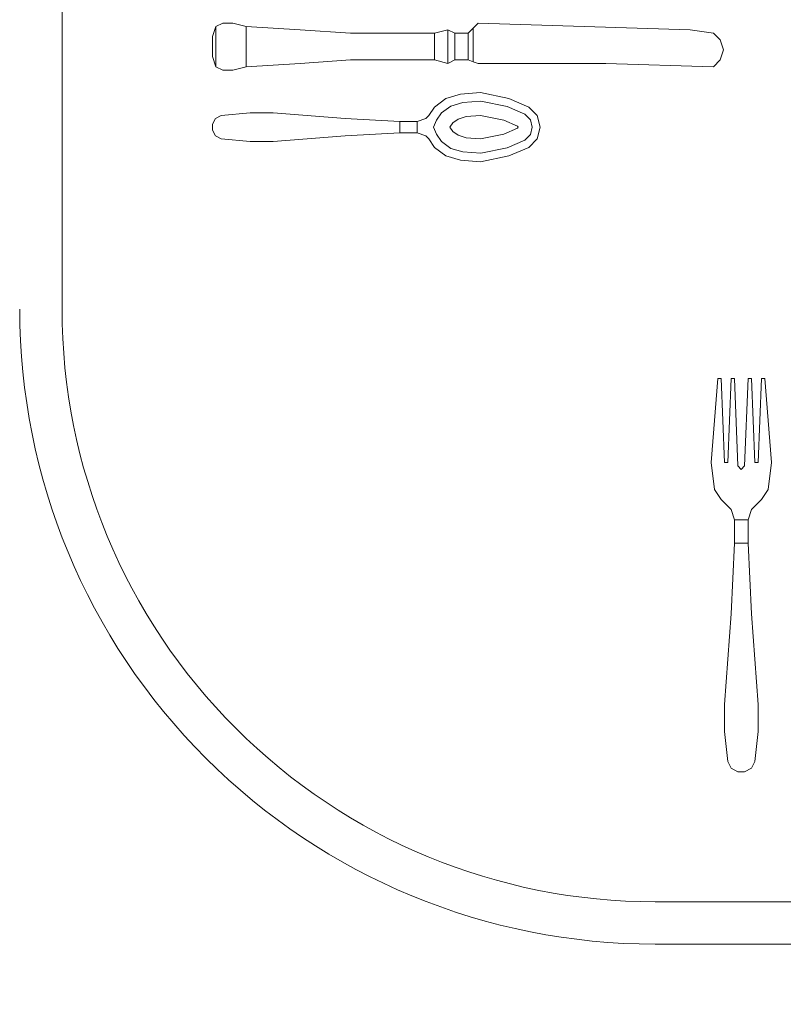
# Model space of a CAD drawing. Units: inches. Extents: x 375 to 1122, y 27 to 1069.
# Tile 85 of 155: x 705.14 to 719.12, y 845.63 to 863.67. Entities that reach past the tile are written whole.
import ezdxf

# ---------------------------------------------------------------- set-up
doc = ezdxf.new("R2010")
doc.units = ezdxf.units.IN
doc.layers.add('A-ANNO-DIMS', color=2, linetype='Continuous', lineweight=18)
doc.layers.add('Furniture', color=30, linetype='Continuous', lineweight=18)
doc.styles.get("Standard").update_dxf_attribs({"font": 'arial.ttf'})
doc.dimstyles.new('ISO-25', dxfattribs={"dimtxt": 12, "dimasz": 2.5, "dimexe": 1.5, "dimexo": 1.5, "dimtad": 1, "dimdec": 1, "dimlunit": 3, "dimtxsty": 'Standard', "dimblk": 'ARCHTICK', "dimcen": 2.5, "dimadec": 0, "dimazin": 0, "dimtfac": 1, "dimtdec": 1, "dimtmove": 0, "dimatfit": 3, "dimfxl": 1.5, "dimfxlon": 1, "dimarcsym": 0})

# ---------------------------------------------------------------- blocks, each defined once
blk = doc.blocks.new('A$C403C54AD')
for p, q in [((2.27071, 1.26108, -0.0006), (2.27071, 0.79569, -0.0006)), ((2.2901, 1.26108, -0.0006), (2.2901, 0.79569, -0.0006)), ((2.08179, 0.82287, -0.05014), (2.08641, 0.82595, -0.04968)), ((2.08179, 0.82287, -0.05322), (2.08641, 0.82595, -0.05276)), ((0.83575, 0.52421, -0.0006), (1.99923, 0.52421, -0.0006))]:
    blk.add_line(p, q)
for radius in [0.27148, 0.29087]:
    blk.add_arc((1.99923, 0.79569, -0.0006), radius, 270, 0)
for points, invisible_edges in [([(2.06948, 0.84288, -0.04954), (2.06948, 0.84903, -0.04954), (2.031, 0.84596, -0.04244), (2.031, 0.84442, -0.04244)], 1), ([(2.06948, 0.84288, -0.05262), (2.06948, 0.84903, -0.05262), (2.031, 0.84596, -0.04552), (2.031, 0.84442, -0.04552)], 1), ([(2.08179, 0.84749, -0.05014), (2.06948, 0.84134, -0.04954), (2.06948, 0.84288, -0.04954), (2.06948, 0.84903, -0.04954)], 5), ([(2.08179, 0.84749, -0.05322), (2.06948, 0.84134, -0.05262), (2.06948, 0.84288, -0.05262), (2.06948, 0.84903, -0.05262)], 5), ([(2.08179, 0.84749, -0.05014), (2.08179, 0.84749, -0.05322), (2.06948, 0.84903, -0.05262), (2.06948, 0.84903, -0.04954)], 1), ([(2.08179, 0.84749, -0.05014), (2.07268, 0.83518, -0.04994), (2.07102, 0.83672, -0.04979), (2.06948, 0.84134, -0.04954)], 13), ([(2.08179, 0.84749, -0.05322), (2.07268, 0.83518, -0.05301), (2.07102, 0.83672, -0.05286), (2.06948, 0.84134, -0.05262)], 13), ([(2.08179, 0.84749, -0.05014), (2.07268, 0.83518, -0.04994), (2.08179, 0.82287, -0.05014), (2.08179, 0.84749, -0.05014)], 7), ([(2.08179, 0.84749, -0.05322), (2.07268, 0.83518, -0.05301), (2.08179, 0.82287, -0.05322), (2.08179, 0.84749, -0.05322)], 7), ([(2.08641, 0.84442, -0.04968), (2.08641, 0.82595, -0.04968), (2.08179, 0.82287, -0.05014), (2.08179, 0.84749, -0.05014)], 5), ([(2.08641, 0.84442, -0.05276), (2.08641, 0.82595, -0.05276), (2.08179, 0.82287, -0.05322), (2.08179, 0.84749, -0.05322)], 5), ([(2.08641, 0.84442, -0.05276), (2.08641, 0.84442, -0.04968), (2.08179, 0.84749, -0.05014), (2.08179, 0.84749, -0.05322)], 4), ([(2.08949, 0.82902, -0.05152), (2.08949, 0.84134, -0.05152), (2.08641, 0.84442, -0.05276), (2.08641, 0.82595, -0.05276)], 5), ([(2.08949, 0.82902, -0.04844), (2.08949, 0.84134, -0.04844), (2.08641, 0.84442, -0.04968), (2.08641, 0.82595, -0.04968)], 5), ([(2.06948, 0.84134, -0.04954), (2.07102, 0.83672, -0.04979), (2.031, 0.83826, -0.04244), (2.031, 0.8398, -0.04244)], 1), ([(2.06948, 0.84134, -0.05262), (2.07102, 0.83672, -0.05286), (2.031, 0.83826, -0.04552), (2.031, 0.8398, -0.04552)], 1), ([(2.09103, 0.83056, -0.04739), (2.09103, 0.8398, -0.04739), (2.08949, 0.84134, -0.04844), (2.08949, 0.82902, -0.04844)], 5), ([(2.09103, 0.83056, -0.05018), (2.09103, 0.8398, -0.05018), (2.08949, 0.84134, -0.05152), (2.08949, 0.82902, -0.05152)], 5), ([(2.09103, 0.8398, -0.05018), (2.09103, 0.8398, -0.04739), (2.08949, 0.84134, -0.04844), (2.08949, 0.84134, -0.05152)], 1), ([(2.09564, 0.83826, -0.04504), (2.09564, 0.8321, -0.04504), (2.09103, 0.83056, -0.04739), (2.09103, 0.8398, -0.04739)], 4), ([(2.09564, 0.83826, -0.04763), (2.09564, 0.8321, -0.04763), (2.09103, 0.83056, -0.05018), (2.09103, 0.8398, -0.05018)], 4), ([(2.09564, 0.83826, -0.04504), (2.09564, 0.83826, -0.04763), (2.09103, 0.8398, -0.05018), (2.09103, 0.8398, -0.04739)], 5), ([(2.13874, 0.8398, -0.04587), (2.13874, 0.83056, -0.04587), (2.10642, 0.8321, -0.04296), (2.10642, 0.83826, -0.04296)], 1), ([(2.13874, 0.8398, -0.04587), (2.13874, 0.8398, -0.04895), (2.10642, 0.83826, -0.04555), (2.10642, 0.83826, -0.04296)], 5), ([(2.13874, 0.8398, -0.04895), (2.13874, 0.83056, -0.04895), (2.10642, 0.8321, -0.04555), (2.10642, 0.83826, -0.04555)], 1), ([(2.1803, 0.82749, -0.04825), (2.1803, 0.84288, -0.04825), (2.13874, 0.8398, -0.04587), (2.13874, 0.83056, -0.04587)], 5), ([(2.1803, 0.82749, -0.05289), (2.1803, 0.84288, -0.05289), (2.13874, 0.8398, -0.04895), (2.13874, 0.83056, -0.04895)], 5), ([(2.1803, 0.84288, -0.05289), (2.1803, 0.84288, -0.04825), (2.13874, 0.8398, -0.04587), (2.13874, 0.8398, -0.04895)], 4), ([(2.19261, 0.84288, -0.04858), (2.19261, 0.82749, -0.04858), (2.1803, 0.82749, -0.04825), (2.1803, 0.84288, -0.04825)], 5), ([(2.19261, 0.84288, -0.05321), (2.19261, 0.82749, -0.05321), (2.1803, 0.82749, -0.05289), (2.1803, 0.84288, -0.05289)], 5), ([(2.20647, 0.82902, -0.04855), (2.20647, 0.84134, -0.04855), (2.19261, 0.84288, -0.04858), (2.19261, 0.82749, -0.04858)], 5), ([(2.20647, 0.82902, -0.05318), (2.20647, 0.84134, -0.05318), (2.19261, 0.84288, -0.05321), (2.19261, 0.82749, -0.05321)], 5), ([(2.20954, 0.8398, -0.0483), (2.20954, 0.83056, -0.0483), (2.20647, 0.82902, -0.04855), (2.20647, 0.84134, -0.04855)], 5), ([(2.20954, 0.8398, -0.05294), (2.20954, 0.83056, -0.05294), (2.20647, 0.82902, -0.05318), (2.20647, 0.84134, -0.05318)], 5), ([(2.21108, 0.83364, -0.04847), (2.21108, 0.83672, -0.04847), (2.20954, 0.8398, -0.0483), (2.20954, 0.83056, -0.0483)], 4), ([(2.21108, 0.83364, -0.0526), (2.21108, 0.83672, -0.0526), (2.20954, 0.8398, -0.05294), (2.20954, 0.83056, -0.05294)], 4), ([(2.08179, 0.82287, -0.05014), (2.07268, 0.83518, -0.04994), (2.07102, 0.83364, -0.04979), (2.06948, 0.82902, -0.04954)], 13), ([(2.08179, 0.82287, -0.05322), (2.07268, 0.83518, -0.05301), (2.07102, 0.83364, -0.05286), (2.06948, 0.82902, -0.05262)], 13), ([(2.10642, 0.83826, -0.04555), (2.10642, 0.83826, -0.04296), (2.09564, 0.83826, -0.04504), (2.09564, 0.83826, -0.04763)], 5), ([(2.07102, 0.83364, -0.04979), (2.06948, 0.82902, -0.04954), (2.031, 0.83056, -0.04244), (2.031, 0.8321, -0.04244)], 1), ([(2.07102, 0.83364, -0.05286), (2.06948, 0.82902, -0.05262), (2.031, 0.83056, -0.04552), (2.031, 0.8321, -0.04552)], 1), ([(2.09103, 0.83056, -0.04739), (2.09103, 0.83056, -0.05018), (2.08949, 0.82902, -0.05152), (2.08949, 0.82902, -0.04844)], 1), ([(2.09564, 0.8321, -0.04763), (2.09564, 0.8321, -0.04504), (2.09103, 0.83056, -0.04739), (2.09103, 0.83056, -0.05018)], 5), ([(2.09564, 0.8321, -0.04763), (2.09564, 0.8321, -0.04504), (2.10642, 0.8321, -0.04296), (2.10642, 0.8321, -0.04555)], 5), ([(2.10642, 0.8321, -0.04296), (2.10642, 0.8321, -0.04555), (2.13874, 0.83056, -0.04895), (2.13874, 0.83056, -0.04587)], 5), ([(2.13874, 0.83056, -0.04895), (2.13874, 0.83056, -0.04587), (2.1803, 0.82749, -0.04825), (2.1803, 0.82749, -0.05289)], 1), ([(1.88505, 0.82556, -0.0249), (1.87581, 0.82556, -0.0249), (1.87273, 0.82248, -0.0249), (1.88813, 0.82248, -0.0249)], 5), ([(1.88505, 0.82556, -0.02644), (1.87581, 0.82556, -0.02644), (1.87273, 0.82248, -0.02644), (1.88813, 0.82248, -0.02644)], 5), ([(1.87581, 0.82556, -0.02644), (1.87581, 0.82556, -0.0249), (1.87273, 0.82248, -0.0249), (1.87273, 0.82248, -0.02644)], 5), ([(1.88043, 0.8271, -0.0249), (1.88043, 0.8271, -0.0249), (1.88505, 0.82556, -0.0249), (1.87581, 0.82556, -0.0249)], 4), ([(1.88043, 0.8271, -0.02644), (1.88043, 0.8271, -0.02644), (1.88505, 0.82556, -0.02644), (1.87581, 0.82556, -0.02644)], 4), ([(1.88043, 0.8271, -0.0249), (1.88043, 0.8271, -0.02644), (1.87581, 0.82556, -0.02644), (1.87581, 0.82556, -0.0249)], 4), ([(1.88505, 0.82556, -0.02644), (1.88505, 0.82556, -0.0249), (1.88043, 0.8271, -0.0249), (1.88043, 0.8271, -0.02644)], 1), ([(1.88813, 0.82248, -0.0249), (1.88813, 0.82248, -0.02644), (1.88505, 0.82556, -0.02644), (1.88505, 0.82556, -0.0249)], 5), ([(2.06948, 0.82749, -0.04954), (2.06948, 0.82133, -0.04954), (2.031, 0.82441, -0.04244), (2.031, 0.82595, -0.04244)], 1), ([(2.06948, 0.82749, -0.05262), (2.06948, 0.82133, -0.05262), (2.031, 0.82441, -0.04552), (2.031, 0.82595, -0.04552)], 1), ([(2.08179, 0.82287, -0.05014), (2.06948, 0.82902, -0.04954), (2.06948, 0.82749, -0.04954), (2.06948, 0.82133, -0.04954)], 5), ([(2.08179, 0.82287, -0.05322), (2.06948, 0.82902, -0.05262), (2.06948, 0.82749, -0.05262), (2.06948, 0.82133, -0.05262)], 5), ([(2.08641, 0.82595, -0.04968), (2.08641, 0.82595, -0.05276), (2.08179, 0.82287, -0.05322), (2.08179, 0.82287, -0.05014)], 4), ([(1.87273, 0.82248, -0.0249), (1.88813, 0.82248, -0.0249), (1.88659, 0.77323, -0.0249), (1.8712, 0.81171, -0.0249)], 5), ([(1.87273, 0.82248, -0.02644), (1.88813, 0.82248, -0.02644), (1.88659, 0.77323, -0.02644), (1.8712, 0.81171, -0.02644)], 5), ([(1.87273, 0.82248, -0.0249), (1.87273, 0.82248, -0.02644), (1.8712, 0.81171, -0.02644), (1.8712, 0.81171, -0.0249)], 5), ([(1.88659, 0.77323, -0.02644), (1.88659, 0.77323, -0.0249), (1.88813, 0.82248, -0.0249), (1.88813, 0.82248, -0.02644)], 5), ([(2.08179, 0.82287, -0.05322), (2.08179, 0.82287, -0.05014), (2.06948, 0.82133, -0.04954), (2.06948, 0.82133, -0.05262)], 1), ([(1.88659, 0.77323, -0.0249), (1.8712, 0.81171, -0.0249), (1.86812, 0.71474, -0.0249), (1.88659, 0.71474, -0.0249)], 5), ([(1.88659, 0.77323, -0.02644), (1.8712, 0.81171, -0.02644), (1.86812, 0.71474, -0.02644), (1.88659, 0.71474, -0.02644)], 5), ([(1.8712, 0.81171, -0.02644), (1.8712, 0.81171, -0.0249), (1.86812, 0.71474, -0.0249), (1.86812, 0.71474, -0.02644)], 5), ([(1.88659, 0.71474, -0.0249), (1.88659, 0.71474, -0.02644), (1.88659, 0.77323, -0.02644), (1.88659, 0.77323, -0.0249)], 5), ([(1.90985, 0.73605, -0.02421), (1.9066, 0.73789, -0.02157), (1.91055, 0.74173, -0.02048), (1.91253, 0.73867, -0.02365)], 5), ([(1.90985, 0.73605, -0.02289), (1.9066, 0.73789, -0.02025), (1.91055, 0.74173, -0.01916), (1.91253, 0.73867, -0.02233)], 5), ([(1.91055, 0.74173, -0.02048), (1.91253, 0.73867, -0.02365), (1.91583, 0.73948, -0.02346), (1.91583, 0.74304, -0.02029)], 5), ([(1.91055, 0.74173, -0.01916), (1.91253, 0.73867, -0.02233), (1.91583, 0.73948, -0.02215), (1.91583, 0.74304, -0.01897)], 5), ([(1.92111, 0.74173, -0.02048), (1.91914, 0.73867, -0.02365), (1.91583, 0.73948, -0.02346), (1.91583, 0.74304, -0.02029)], 5), ([(1.92111, 0.74173, -0.01916), (1.91914, 0.73867, -0.02233), (1.91583, 0.73948, -0.02215), (1.91583, 0.74304, -0.01897)], 5), ([(1.92182, 0.73605, -0.02421), (1.92507, 0.73789, -0.02157), (1.92111, 0.74173, -0.02048), (1.91914, 0.73867, -0.02365)], 5), ([(1.92182, 0.73605, -0.02289), (1.92507, 0.73789, -0.02025), (1.92111, 0.74173, -0.01916), (1.91914, 0.73867, -0.02233)], 5), ([(1.90264, 0.72882, -0.0234), (1.90634, 0.72802, -0.02592), (1.90985, 0.73605, -0.02421), (1.9066, 0.73789, -0.02157)], 5), ([(1.90264, 0.72882, -0.02208), (1.90634, 0.72802, -0.0246), (1.90985, 0.73605, -0.02289), (1.9066, 0.73789, -0.02025)], 5), ([(1.90985, 0.73605, -0.02421), (1.9154, 0.73267, -0.0271), (1.91266, 0.72644, -0.02873), (1.90634, 0.72802, -0.02592)], 5), ([(1.90985, 0.73605, -0.02289), (1.9154, 0.73267, -0.02578), (1.91266, 0.72644, -0.02741), (1.90634, 0.72802, -0.0246)], 5), ([(1.9154, 0.73267, -0.02578), (1.91253, 0.73867, -0.02233), (1.90985, 0.73605, -0.02289), (1.9154, 0.73267, -0.02578)], 5), ([(1.9154, 0.73267, -0.0271), (1.91253, 0.73867, -0.02365), (1.90985, 0.73605, -0.02421), (1.9154, 0.73267, -0.0271)], 5), ([(1.91583, 0.73948, -0.02215), (1.91583, 0.73309, -0.02564), (1.9154, 0.73267, -0.02578), (1.91253, 0.73867, -0.02233)], 5), ([(1.91583, 0.73948, -0.02346), (1.91583, 0.73309, -0.02696), (1.9154, 0.73267, -0.0271), (1.91253, 0.73867, -0.02365)], 5), ([(1.91583, 0.73948, -0.02215), (1.91583, 0.73309, -0.02564), (1.91627, 0.73267, -0.02578), (1.91914, 0.73867, -0.02233)], 5), ([(1.91583, 0.73948, -0.02346), (1.91583, 0.73309, -0.02696), (1.91627, 0.73267, -0.0271), (1.91914, 0.73867, -0.02365)], 5), ([(1.91627, 0.73267, -0.02578), (1.91914, 0.73867, -0.02233), (1.92182, 0.73605, -0.02289), (1.91627, 0.73267, -0.02578)], 5), ([(1.91627, 0.73267, -0.0271), (1.91914, 0.73867, -0.02365), (1.92182, 0.73605, -0.02421), (1.91627, 0.73267, -0.0271)], 5), ([(1.92182, 0.73605, -0.02421), (1.91627, 0.73267, -0.0271), (1.91901, 0.72644, -0.02873), (1.92532, 0.72802, -0.02592)], 5), ([(1.92182, 0.73605, -0.02289), (1.91627, 0.73267, -0.02578), (1.91901, 0.72644, -0.02741), (1.92532, 0.72802, -0.0246)], 5), ([(1.92903, 0.72882, -0.0234), (1.92532, 0.72802, -0.02592), (1.92182, 0.73605, -0.02421), (1.92507, 0.73789, -0.02157)], 5), ([(1.92903, 0.72882, -0.02208), (1.92532, 0.72802, -0.0246), (1.92182, 0.73605, -0.02289), (1.92507, 0.73789, -0.02025)], 5), ([(1.9154, 0.73267, -0.0271), (1.91627, 0.73267, -0.0271), (1.91901, 0.72644, -0.02873), (1.91266, 0.72644, -0.02873)], 5), ([(1.9154, 0.73267, -0.02578), (1.91627, 0.73267, -0.02578), (1.91901, 0.72644, -0.02741), (1.91266, 0.72644, -0.02741)], 5), ([(1.91583, 0.73309, -0.02564), (1.91627, 0.73267, -0.02578), (1.9154, 0.73267, -0.02578), (1.91583, 0.73309, -0.02564)], 2), ([(1.91583, 0.73309, -0.02696), (1.91627, 0.73267, -0.0271), (1.9154, 0.73267, -0.0271), (1.91583, 0.73309, -0.02696)], 2), ([(1.90388, 0.71589, -0.0279), (1.9, 0.71579, -0.02544), (1.90264, 0.72882, -0.0234), (1.90634, 0.72802, -0.02592)], 5), ([(1.90388, 0.71589, -0.02658), (1.9, 0.71579, -0.02412), (1.90264, 0.72882, -0.02208), (1.90634, 0.72802, -0.0246)], 5), ([(1.91266, 0.72644, -0.02741), (1.90634, 0.72802, -0.0246), (1.90388, 0.71589, -0.02658), (1.91051, 0.71583, -0.02912)], 5), ([(1.91266, 0.72644, -0.02873), (1.90634, 0.72802, -0.02592), (1.90388, 0.71589, -0.0279), (1.91051, 0.71583, -0.03044)], 5), ([(1.91901, 0.72644, -0.02741), (1.91266, 0.72644, -0.02741), (1.91051, 0.71583, -0.02912), (1.92116, 0.71583, -0.02912)], 5), ([(1.91901, 0.72644, -0.02873), (1.91266, 0.72644, -0.02873), (1.91051, 0.71583, -0.03044), (1.92116, 0.71583, -0.03044)], 5), ([(1.91901, 0.72644, -0.02741), (1.92532, 0.72802, -0.0246), (1.92778, 0.71589, -0.02658), (1.92116, 0.71583, -0.02912)], 5), ([(1.91901, 0.72644, -0.02873), (1.92532, 0.72802, -0.02592), (1.92778, 0.71589, -0.0279), (1.92116, 0.71583, -0.03044)], 5), ([(1.92778, 0.71589, -0.0279), (1.93166, 0.71579, -0.02544), (1.92903, 0.72882, -0.0234), (1.92532, 0.72802, -0.02592)], 5), ([(1.92778, 0.71589, -0.02658), (1.93166, 0.71579, -0.02412), (1.92903, 0.72882, -0.02208), (1.92532, 0.72802, -0.0246)], 5), ([(1.86812, 0.71474, -0.0249), (1.88659, 0.71474, -0.0249), (1.88582, 0.71243, -0.02413), (1.87043, 0.71243, -0.02413)], 1), ([(1.86812, 0.71474, -0.02644), (1.88659, 0.71474, -0.02644), (1.88582, 0.71243, -0.02721), (1.87043, 0.71243, -0.02721)], 1), ([(1.86812, 0.71474, -0.02644), (1.86812, 0.71474, -0.0249), (1.87043, 0.71243, -0.02413), (1.87043, 0.71243, -0.02721)], 5), ([(1.88582, 0.71243, -0.02721), (1.88582, 0.71243, -0.02413), (1.88659, 0.71474, -0.0249), (1.88659, 0.71474, -0.02644)], 5), ([(1.90066, 0.70658, -0.02499), (1.90447, 0.70765, -0.02747), (1.90388, 0.71589, -0.02658), (1.9, 0.71579, -0.02412)], 5), ([(1.90066, 0.70658, -0.02631), (1.90447, 0.70765, -0.02879), (1.90388, 0.71589, -0.0279), (1.9, 0.71579, -0.02544)], 5), ([(1.90388, 0.71589, -0.0279), (1.91051, 0.71583, -0.03044), (1.91098, 0.70922, -0.03139), (1.90447, 0.70765, -0.02879)], 5), ([(1.90388, 0.71589, -0.02658), (1.91051, 0.71583, -0.02912), (1.91098, 0.70922, -0.03007), (1.90447, 0.70765, -0.02747)], 5), ([(1.91051, 0.71583, -0.03044), (1.92116, 0.71583, -0.03044), (1.92068, 0.70922, -0.03139), (1.91098, 0.70922, -0.03139)], 5), ([(1.91051, 0.71583, -0.02912), (1.92116, 0.71583, -0.02912), (1.92068, 0.70922, -0.03007), (1.91098, 0.70922, -0.03007)], 5), ([(1.92778, 0.71589, -0.0279), (1.92116, 0.71583, -0.03044), (1.92068, 0.70922, -0.03139), (1.92719, 0.70765, -0.02879)], 5), ([(1.92778, 0.71589, -0.02658), (1.92116, 0.71583, -0.02912), (1.92068, 0.70922, -0.03007), (1.92719, 0.70765, -0.02747)], 5), ([(1.931, 0.70658, -0.02499), (1.92719, 0.70765, -0.02747), (1.92778, 0.71589, -0.02658), (1.93166, 0.71579, -0.02412)], 5), ([(1.931, 0.70658, -0.02631), (1.92719, 0.70765, -0.02879), (1.92778, 0.71589, -0.0279), (1.93166, 0.71579, -0.02544)], 5), ([(1.87043, 0.71243, -0.02413), (1.87043, 0.71243, -0.02721), (1.87273, 0.71012, -0.03029), (1.87273, 0.71012, -0.02105)], 5), ([(1.87273, 0.71012, -0.03029), (1.87273, 0.71012, -0.02105), (1.87273, 0.70396, -0.02105), (1.87273, 0.70396, -0.03029)], 1), ([(1.88505, 0.71012, -0.02105), (1.88505, 0.71012, -0.03029), (1.88582, 0.71243, -0.02721), (1.88582, 0.71243, -0.02413)], 5), ([(1.88505, 0.70396, -0.03029), (1.88505, 0.70396, -0.02105), (1.88505, 0.71012, -0.02105), (1.88505, 0.71012, -0.03029)], 4), ([(1.91098, 0.70922, -0.03007), (1.90447, 0.70765, -0.02747), (1.90613, 0.70213, -0.02798), (1.9121, 0.7055, -0.0303)], 5), ([(1.92068, 0.70922, -0.03139), (1.91098, 0.70922, -0.03139), (1.9121, 0.7055, -0.03162), (1.91956, 0.7055, -0.03162)], 5), ([(1.92068, 0.70922, -0.03007), (1.91098, 0.70922, -0.03007), (1.9121, 0.7055, -0.0303), (1.91956, 0.7055, -0.0303)], 5), ([(1.92068, 0.70922, -0.03139), (1.92719, 0.70765, -0.02879), (1.92553, 0.70213, -0.0293), (1.91956, 0.7055, -0.03162)], 5), ([(1.92068, 0.70922, -0.03007), (1.92719, 0.70765, -0.02747), (1.92553, 0.70213, -0.02798), (1.91956, 0.7055, -0.0303)], 5), ([(1.90613, 0.70213, -0.02798), (1.90264, 0.69998, -0.02539), (1.90066, 0.70658, -0.02499), (1.90447, 0.70765, -0.02747)], 5), ([(1.90613, 0.70213, -0.0293), (1.90264, 0.69998, -0.02671), (1.90066, 0.70658, -0.02631), (1.90447, 0.70765, -0.02879)], 5), ([(1.90613, 0.70213, -0.0293), (1.9121, 0.7055, -0.03162), (1.91387, 0.70313, -0.03172), (1.90928, 0.69791, -0.02947)], 5), ([(1.90613, 0.70213, -0.02798), (1.9121, 0.7055, -0.0303), (1.91387, 0.70313, -0.0304), (1.90928, 0.69791, -0.02815)], 5), ([(1.9121, 0.7055, -0.03162), (1.91956, 0.7055, -0.03162), (1.91779, 0.70313, -0.03172), (1.91387, 0.70313, -0.03172)], 5), ([(1.9121, 0.7055, -0.0303), (1.91956, 0.7055, -0.0303), (1.91779, 0.70313, -0.0304), (1.91387, 0.70313, -0.0304)], 5), ([(1.92553, 0.70213, -0.0293), (1.91956, 0.7055, -0.03162), (1.91779, 0.70313, -0.03172), (1.92238, 0.69791, -0.02947)], 5), ([(1.92553, 0.70213, -0.02798), (1.91956, 0.7055, -0.0303), (1.91779, 0.70313, -0.0304), (1.92238, 0.69791, -0.02815)], 5), ([(1.92553, 0.70213, -0.02798), (1.92903, 0.69998, -0.02539), (1.931, 0.70658, -0.02499), (1.92719, 0.70765, -0.02747)], 5), ([(1.92553, 0.70213, -0.0293), (1.92903, 0.69998, -0.02671), (1.931, 0.70658, -0.02631), (1.92719, 0.70765, -0.02879)], 5), ([(1.9066, 0.69472, -0.02719), (1.90928, 0.69791, -0.02947), (1.90613, 0.70213, -0.0293), (1.90264, 0.69998, -0.02671)], 5), ([(1.9066, 0.69472, -0.02588), (1.90928, 0.69791, -0.02815), (1.90613, 0.70213, -0.02798), (1.90264, 0.69998, -0.02539)], 5), ([(1.91387, 0.70313, -0.03172), (1.90928, 0.69791, -0.02947), (1.91269, 0.69562, -0.02948), (1.91583, 0.70178, -0.03152)], 5), ([(1.91387, 0.70313, -0.0304), (1.90928, 0.69791, -0.02815), (1.91269, 0.69562, -0.02816), (1.91583, 0.70178, -0.0302)], 5), ([(1.91269, 0.69562, -0.02948), (1.91583, 0.70178, -0.03152), (1.91583, 0.70178, -0.03152), (1.91583, 0.69426, -0.0293)], 5), ([(1.91269, 0.69562, -0.02816), (1.91583, 0.70178, -0.0302), (1.91583, 0.70178, -0.0302), (1.91583, 0.69426, -0.02798)], 5), ([(1.91779, 0.70313, -0.03172), (1.91387, 0.70313, -0.03172), (1.91583, 0.70178, -0.03152)], 1), ([(1.91779, 0.70313, -0.0304), (1.91387, 0.70313, -0.0304), (1.91583, 0.70178, -0.0302)], 1), ([(1.91779, 0.70313, -0.03172), (1.92238, 0.69791, -0.02947), (1.91897, 0.69562, -0.02948), (1.91583, 0.70178, -0.03152)], 5), ([(1.91779, 0.70313, -0.0304), (1.92238, 0.69791, -0.02815), (1.91897, 0.69562, -0.02816), (1.91583, 0.70178, -0.0302)], 5), ([(1.91897, 0.69562, -0.02948), (1.91583, 0.70178, -0.03152), (1.91583, 0.70178, -0.03152), (1.91583, 0.69426, -0.0293)], 5), ([(1.91897, 0.69562, -0.02816), (1.91583, 0.70178, -0.0302), (1.91583, 0.70178, -0.0302), (1.91583, 0.69426, -0.02798)], 5), ([(1.92507, 0.69472, -0.02719), (1.92238, 0.69791, -0.02947), (1.92553, 0.70213, -0.0293), (1.92903, 0.69998, -0.02671)], 5), ([(1.92507, 0.69472, -0.02588), (1.92238, 0.69791, -0.02815), (1.92553, 0.70213, -0.02798), (1.92903, 0.69998, -0.02539)], 5), ([(1.87273, 0.69473, -0.02105), (1.88505, 0.69473, -0.02105), (1.88505, 0.65625, -0.01951), (1.87273, 0.65625, -0.01951)], 4), ([(1.87273, 0.69473, -0.03029), (1.88505, 0.69473, -0.03029), (1.88505, 0.65625, -0.03183), (1.87273, 0.65625, -0.03183)], 4), ([(1.91269, 0.69562, -0.02816), (1.91055, 0.6921, -0.02625), (1.9066, 0.69472, -0.02588), (1.90928, 0.69791, -0.02815)], 5), ([(1.91055, 0.6921, -0.0284), (1.91583, 0.6921, -0.0284), (1.91583, 0.69426, -0.0293), (1.91269, 0.69562, -0.02948)], 11), ([(1.91055, 0.6921, -0.02625), (1.91583, 0.6921, -0.02625), (1.91583, 0.69426, -0.02798), (1.91269, 0.69562, -0.02816)], 11), ([(1.92111, 0.6921, -0.0284), (1.91583, 0.6921, -0.0284), (1.91583, 0.69426, -0.0293), (1.91897, 0.69562, -0.02948)], 11), ([(1.92111, 0.6921, -0.02625), (1.91583, 0.6921, -0.02625), (1.91583, 0.69426, -0.02798), (1.91897, 0.69562, -0.02816)], 11), ([(1.91897, 0.69562, -0.02948), (1.92111, 0.6921, -0.0284), (1.92507, 0.69472, -0.02719), (1.92238, 0.69791, -0.02947)], 5), ([(1.91897, 0.69562, -0.02816), (1.92111, 0.6921, -0.02625), (1.92507, 0.69472, -0.02588), (1.92238, 0.69791, -0.02815)], 5), ([(1.91187, 0.69077, -0.02551), (1.91979, 0.69077, -0.02551), (1.92111, 0.6921, -0.02625), (1.91055, 0.6921, -0.02625)], 5), ([(1.91187, 0.69077, -0.0276), (1.91979, 0.69077, -0.0276), (1.92111, 0.6921, -0.0284), (1.91055, 0.6921, -0.0284)], 5), ([(1.91187, 0.69077, -0.02551), (1.91187, 0.69077, -0.0276), (1.91055, 0.6921, -0.0284), (1.91055, 0.6921, -0.02625)], 1), ([(1.91847, 0.68681, -0.02366), (1.91319, 0.68681, -0.02366), (1.91187, 0.69077, -0.02551), (1.91979, 0.69077, -0.02551)], 4), ([(1.91319, 0.68681, -0.02588), (1.91319, 0.68681, -0.02366), (1.91187, 0.69077, -0.02551), (1.91187, 0.69077, -0.0276)], 5), ([(1.91847, 0.68681, -0.02588), (1.91319, 0.68681, -0.02588), (1.91187, 0.69077, -0.0276), (1.91979, 0.69077, -0.0276)], 4), ([(1.91847, 0.68681, -0.02366), (1.91847, 0.68681, -0.02588), (1.91979, 0.69077, -0.0276), (1.91979, 0.69077, -0.02551)], 5), ([(1.91979, 0.69077, -0.0276), (1.91979, 0.69077, -0.02551), (1.92111, 0.6921, -0.02625), (1.92111, 0.6921, -0.0284)], 1), ([(1.91319, 0.68681, -0.02588), (1.91319, 0.68681, -0.02366), (1.91319, 0.6789, -0.02303), (1.91319, 0.6789, -0.02525)], 5), ([(1.91847, 0.6789, -0.02525), (1.91847, 0.6789, -0.02303), (1.91847, 0.68681, -0.02366), (1.91847, 0.68681, -0.02588)], 5), ([(1.91979, 0.65383, -0.02553), (1.91187, 0.65383, -0.02553), (1.91319, 0.6789, -0.02303), (1.91847, 0.6789, -0.02303)], 1), ([(1.91319, 0.6789, -0.02303), (1.91319, 0.6789, -0.02525), (1.91187, 0.65383, -0.02816), (1.91187, 0.65383, -0.02553)], 5), ([(1.91979, 0.65383, -0.02816), (1.91187, 0.65383, -0.02816), (1.91319, 0.6789, -0.02525), (1.91847, 0.6789, -0.02525)], 1), ([(1.91979, 0.65383, -0.02553), (1.91979, 0.65383, -0.02816), (1.91847, 0.6789, -0.02525), (1.91847, 0.6789, -0.02303)], 5), ([(1.88505, 0.65625, -0.01951), (1.87273, 0.65625, -0.01951), (1.8712, 0.63316, -0.01951), (1.88659, 0.63316, -0.01951)], 5), ([(1.88505, 0.65625, -0.03183), (1.87273, 0.65625, -0.03183), (1.8712, 0.63316, -0.03183), (1.88659, 0.63316, -0.03183)], 5), ([(1.90924, 0.62085, -0.03154), (1.92243, 0.62085, -0.03154), (1.91979, 0.65383, -0.02816), (1.91187, 0.65383, -0.02816)], 5), ([(1.91187, 0.65383, -0.02816), (1.91187, 0.65383, -0.02553), (1.90924, 0.62085, -0.02757), (1.90924, 0.62085, -0.03154)], 1), ([(1.90924, 0.62085, -0.02757), (1.92243, 0.62085, -0.02757), (1.91979, 0.65383, -0.02553), (1.91187, 0.65383, -0.02553)], 5), ([(1.92243, 0.62085, -0.03154), (1.92243, 0.62085, -0.02757), (1.91979, 0.65383, -0.02553), (1.91979, 0.65383, -0.02816)], 4), ([(1.8712, 0.63316, -0.01951), (1.88659, 0.63316, -0.01951), (1.88813, 0.60854, -0.02105), (1.86966, 0.60854, -0.02105)], 1), ([(1.8712, 0.63316, -0.03183), (1.88659, 0.63316, -0.03183), (1.88813, 0.60854, -0.03029), (1.86966, 0.60854, -0.03029)], 1), ([(1.92243, 0.61029, -0.02785), (1.90924, 0.61029, -0.02785), (1.90924, 0.62085, -0.02757), (1.92243, 0.62085, -0.02757)], 5), ([(1.92243, 0.61029, -0.03182), (1.90924, 0.61029, -0.03182), (1.90924, 0.62085, -0.03154), (1.92243, 0.62085, -0.03154)], 5), ([(1.91055, 0.5971, -0.02782), (1.92111, 0.5971, -0.02782), (1.92243, 0.61029, -0.02785), (1.90924, 0.61029, -0.02785)], 5), ([(1.91055, 0.5971, -0.03179), (1.92111, 0.5971, -0.03179), (1.92243, 0.61029, -0.03182), (1.90924, 0.61029, -0.03182)], 5), ([(1.88813, 0.60854, -0.02105), (1.86966, 0.60854, -0.02105), (1.86812, 0.60238, -0.01951), (1.88967, 0.60238, -0.01951)], 4), ([(1.88813, 0.60854, -0.03029), (1.86966, 0.60854, -0.03029), (1.86812, 0.60238, -0.03183), (1.88967, 0.60238, -0.03183)], 4), ([(1.86812, 0.60238, -0.01951), (1.88967, 0.60238, -0.01951), (1.88967, 0.59776, -0.02105), (1.86812, 0.59776, -0.02105)], 5), ([(1.86812, 0.60238, -0.03183), (1.88967, 0.60238, -0.03183), (1.88967, 0.59776, -0.03029), (1.86812, 0.59776, -0.03029)], 5), ([(1.88967, 0.59776, -0.02105), (1.86812, 0.59776, -0.02105), (1.86966, 0.59468, -0.02259), (1.88813, 0.59468, -0.02259)], 1), ([(1.88967, 0.59776, -0.03029), (1.86812, 0.59776, -0.03029), (1.86966, 0.59468, -0.02875), (1.88813, 0.59468, -0.02875)], 1), ([(1.91979, 0.59446, -0.02761), (1.91187, 0.59446, -0.02761), (1.91055, 0.5971, -0.02782), (1.92111, 0.5971, -0.02782)], 5), ([(1.91979, 0.59446, -0.03158), (1.91187, 0.59446, -0.03158), (1.91055, 0.5971, -0.03179), (1.92111, 0.5971, -0.03179)], 5), ([(1.91451, 0.59314, -0.02775), (1.91715, 0.59314, -0.02775), (1.91979, 0.59446, -0.02761), (1.91187, 0.59446, -0.02761)], 4), ([(1.91451, 0.59314, -0.0313), (1.91715, 0.59314, -0.0313), (1.91979, 0.59446, -0.03158), (1.91187, 0.59446, -0.03158)], 4)]:
    blk.add_3dface(points, dxfattribs=dict(invisible_edges=invisible_edges))
for points in [[(2.06948, 0.84903, -0.05262), (2.06948, 0.84903, -0.04954), (2.031, 0.84596, -0.04244), (2.031, 0.84596, -0.04552)], [(2.031, 0.84596, -0.04552), (2.031, 0.84596, -0.04244), (2.031, 0.84442, -0.04244), (2.031, 0.84442, -0.04552)], [(2.031, 0.84442, -0.04244), (2.031, 0.84442, -0.04552), (2.06948, 0.84288, -0.05262), (2.06948, 0.84288, -0.04954)], [(2.08949, 0.84134, -0.04844), (2.08949, 0.84134, -0.05152), (2.08641, 0.84442, -0.05276), (2.08641, 0.84442, -0.04968)], [(2.06948, 0.84134, -0.05262), (2.06948, 0.84134, -0.04954), (2.031, 0.8398, -0.04244), (2.031, 0.8398, -0.04552)], [(2.031, 0.8398, -0.04552), (2.031, 0.8398, -0.04244), (2.031, 0.83826, -0.04244), (2.031, 0.83826, -0.04552)], [(2.06948, 0.84134, -0.05262), (2.06948, 0.84134, -0.04954), (2.06948, 0.84288, -0.04954), (2.06948, 0.84288, -0.05262)], [(2.19261, 0.84288, -0.04858), (2.19261, 0.84288, -0.05321), (2.1803, 0.84288, -0.05289), (2.1803, 0.84288, -0.04825)], [(2.20647, 0.84134, -0.05318), (2.20647, 0.84134, -0.04855), (2.19261, 0.84288, -0.04858), (2.19261, 0.84288, -0.05321)], [(2.20954, 0.8398, -0.0483), (2.20954, 0.8398, -0.05294), (2.20647, 0.84134, -0.05318), (2.20647, 0.84134, -0.04855)], [(2.21108, 0.83672, -0.0526), (2.21108, 0.83672, -0.04847), (2.20954, 0.8398, -0.0483), (2.20954, 0.8398, -0.05294)], [(2.031, 0.83826, -0.04552), (2.031, 0.83826, -0.04244), (2.07102, 0.83672, -0.04979), (2.07102, 0.83672, -0.05286)], [(2.07268, 0.83518, -0.05301), (2.07268, 0.83518, -0.04994), (2.07102, 0.83672, -0.04979), (2.07102, 0.83672, -0.05286)], [(2.07102, 0.83364, -0.04979), (2.07102, 0.83364, -0.05286), (2.07268, 0.83518, -0.05301), (2.07268, 0.83518, -0.04994)], [(2.10642, 0.8321, -0.04296), (2.10642, 0.83826, -0.04296), (2.09564, 0.83826, -0.04504), (2.09564, 0.8321, -0.04504)], [(2.10642, 0.8321, -0.04555), (2.10642, 0.83826, -0.04555), (2.09564, 0.83826, -0.04763), (2.09564, 0.8321, -0.04763)], [(2.21108, 0.83364, -0.04847), (2.21108, 0.83364, -0.0526), (2.21108, 0.83672, -0.0526), (2.21108, 0.83672, -0.04847)], [(2.07102, 0.83364, -0.05286), (2.07102, 0.83364, -0.04979), (2.031, 0.8321, -0.04244), (2.031, 0.8321, -0.04552)], [(2.031, 0.8321, -0.04552), (2.031, 0.8321, -0.04244), (2.031, 0.83056, -0.04244), (2.031, 0.83056, -0.04552)], [(2.031, 0.83056, -0.04244), (2.031, 0.83056, -0.04552), (2.06948, 0.82902, -0.05262), (2.06948, 0.82902, -0.04954)], [(2.20647, 0.82902, -0.04855), (2.20647, 0.82902, -0.05318), (2.20954, 0.83056, -0.05294), (2.20954, 0.83056, -0.0483)], [(2.20954, 0.83056, -0.05294), (2.20954, 0.83056, -0.0483), (2.21108, 0.83364, -0.04847), (2.21108, 0.83364, -0.0526)], [(2.06948, 0.82749, -0.04954), (2.06948, 0.82749, -0.05262), (2.031, 0.82595, -0.04552), (2.031, 0.82595, -0.04244)], [(2.031, 0.82595, -0.04552), (2.031, 0.82595, -0.04244), (2.031, 0.82441, -0.04244), (2.031, 0.82441, -0.04552)], [(2.06948, 0.82749, -0.04954), (2.06948, 0.82749, -0.05262), (2.06948, 0.82902, -0.05262), (2.06948, 0.82902, -0.04954)], [(2.08949, 0.82902, -0.05152), (2.08949, 0.82902, -0.04844), (2.08641, 0.82595, -0.04968), (2.08641, 0.82595, -0.05276)], [(2.1803, 0.82749, -0.04825), (2.1803, 0.82749, -0.05289), (2.19261, 0.82749, -0.05321), (2.19261, 0.82749, -0.04858)], [(2.19261, 0.82749, -0.05321), (2.19261, 0.82749, -0.04858), (2.20647, 0.82902, -0.04855), (2.20647, 0.82902, -0.05318)], [(2.031, 0.82441, -0.04244), (2.031, 0.82441, -0.04552), (2.06948, 0.82133, -0.05262), (2.06948, 0.82133, -0.04954)], [(1.91055, 0.74173, -0.01916), (1.91055, 0.74173, -0.02048), (1.9066, 0.73789, -0.02157), (1.9066, 0.73789, -0.02025)], [(1.91583, 0.74304, -0.02029), (1.91583, 0.74304, -0.01897), (1.91055, 0.74173, -0.01916), (1.91055, 0.74173, -0.02048)], [(1.92111, 0.74173, -0.01916), (1.92111, 0.74173, -0.02048), (1.91583, 0.74304, -0.02029), (1.91583, 0.74304, -0.01897)], [(1.92507, 0.73789, -0.02157), (1.92507, 0.73789, -0.02025), (1.92111, 0.74173, -0.01916), (1.92111, 0.74173, -0.02048)], [(1.9066, 0.73789, -0.02157), (1.9066, 0.73789, -0.02025), (1.90264, 0.72882, -0.02208), (1.90264, 0.72882, -0.0234)], [(1.92903, 0.72882, -0.02208), (1.92903, 0.72882, -0.0234), (1.92507, 0.73789, -0.02157), (1.92507, 0.73789, -0.02025)], [(1.90264, 0.72882, -0.02208), (1.90264, 0.72882, -0.0234), (1.9, 0.71579, -0.02544), (1.9, 0.71579, -0.02412)], [(1.93166, 0.71579, -0.02544), (1.93166, 0.71579, -0.02412), (1.92903, 0.72882, -0.02208), (1.92903, 0.72882, -0.0234)], [(1.9, 0.71579, -0.02544), (1.9, 0.71579, -0.02412), (1.90066, 0.70658, -0.02499), (1.90066, 0.70658, -0.02631)], [(1.931, 0.70658, -0.02499), (1.931, 0.70658, -0.02631), (1.93166, 0.71579, -0.02544), (1.93166, 0.71579, -0.02412)], [(1.87043, 0.71243, -0.02413), (1.88582, 0.71243, -0.02413), (1.88505, 0.71012, -0.02105), (1.87273, 0.71012, -0.02105)], [(1.87043, 0.71243, -0.02721), (1.88582, 0.71243, -0.02721), (1.88505, 0.71012, -0.03029), (1.87273, 0.71012, -0.03029)], [(1.88505, 0.71012, -0.02105), (1.87273, 0.71012, -0.02105), (1.87273, 0.70396, -0.02105), (1.88505, 0.70396, -0.02105)], [(1.88505, 0.71012, -0.03029), (1.87273, 0.71012, -0.03029), (1.87273, 0.70396, -0.03029), (1.88505, 0.70396, -0.03029)], [(1.87273, 0.70396, -0.02105), (1.88505, 0.70396, -0.02105), (1.88659, 0.70089, -0.01951), (1.8712, 0.70089, -0.01951)], [(1.87273, 0.70396, -0.03029), (1.88505, 0.70396, -0.03029), (1.88659, 0.70089, -0.03183), (1.8712, 0.70089, -0.03183)], [(1.87273, 0.70396, -0.02105), (1.87273, 0.70396, -0.03029), (1.8712, 0.70089, -0.03183), (1.8712, 0.70089, -0.01951)], [(1.88659, 0.70089, -0.01951), (1.88659, 0.70089, -0.03183), (1.88505, 0.70396, -0.03029), (1.88505, 0.70396, -0.02105)], [(1.90066, 0.70658, -0.02631), (1.90066, 0.70658, -0.02499), (1.90264, 0.69998, -0.02539), (1.90264, 0.69998, -0.02671)], [(1.92903, 0.69998, -0.02671), (1.92903, 0.69998, -0.02539), (1.931, 0.70658, -0.02499), (1.931, 0.70658, -0.02631)], [(1.88659, 0.70089, -0.01951), (1.8712, 0.70089, -0.01951), (1.87273, 0.69473, -0.02105), (1.88505, 0.69473, -0.02105)], [(1.88659, 0.70089, -0.03183), (1.8712, 0.70089, -0.03183), (1.87273, 0.69473, -0.03029), (1.88505, 0.69473, -0.03029)], [(1.8712, 0.70089, -0.03183), (1.8712, 0.70089, -0.01951), (1.87273, 0.69473, -0.02105), (1.87273, 0.69473, -0.03029)], [(1.88505, 0.69473, -0.03029), (1.88505, 0.69473, -0.02105), (1.88659, 0.70089, -0.01951), (1.88659, 0.70089, -0.03183)], [(1.90264, 0.69998, -0.02539), (1.90264, 0.69998, -0.02671), (1.9066, 0.69472, -0.02719), (1.9066, 0.69472, -0.02588)], [(1.92507, 0.69472, -0.02588), (1.92507, 0.69472, -0.02719), (1.92903, 0.69998, -0.02671), (1.92903, 0.69998, -0.02539)], [(1.87273, 0.69473, -0.02105), (1.87273, 0.69473, -0.03029), (1.87273, 0.65625, -0.03183), (1.87273, 0.65625, -0.01951)], [(1.88505, 0.65625, -0.01951), (1.88505, 0.65625, -0.03183), (1.88505, 0.69473, -0.03029), (1.88505, 0.69473, -0.02105)], [(1.9066, 0.69472, -0.02719), (1.9066, 0.69472, -0.02588), (1.91055, 0.6921, -0.02625), (1.91055, 0.6921, -0.0284)], [(1.92111, 0.6921, -0.0284), (1.92111, 0.6921, -0.02625), (1.92507, 0.69472, -0.02588), (1.92507, 0.69472, -0.02719)], [(1.91319, 0.6789, -0.02525), (1.91847, 0.6789, -0.02525), (1.91847, 0.68681, -0.02588), (1.91319, 0.68681, -0.02588)], [(1.91319, 0.6789, -0.02303), (1.91847, 0.6789, -0.02303), (1.91847, 0.68681, -0.02366), (1.91319, 0.68681, -0.02366)], [(1.87273, 0.65625, -0.03183), (1.87273, 0.65625, -0.01951), (1.8712, 0.63316, -0.01951), (1.8712, 0.63316, -0.03183)], [(1.88659, 0.63316, -0.03183), (1.88659, 0.63316, -0.01951), (1.88505, 0.65625, -0.01951), (1.88505, 0.65625, -0.03183)], [(1.8712, 0.63316, -0.01951), (1.8712, 0.63316, -0.03183), (1.86966, 0.60854, -0.03029), (1.86966, 0.60854, -0.02105)], [(1.88813, 0.60854, -0.02105), (1.88813, 0.60854, -0.03029), (1.88659, 0.63316, -0.03183), (1.88659, 0.63316, -0.01951)], [(1.90924, 0.62085, -0.02757), (1.90924, 0.62085, -0.03154), (1.90924, 0.61029, -0.03182), (1.90924, 0.61029, -0.02785)], [(1.92243, 0.61029, -0.02785), (1.92243, 0.61029, -0.03182), (1.92243, 0.62085, -0.03154), (1.92243, 0.62085, -0.02757)], [(1.90924, 0.61029, -0.03182), (1.90924, 0.61029, -0.02785), (1.91055, 0.5971, -0.02782), (1.91055, 0.5971, -0.03179)], [(1.92111, 0.5971, -0.03179), (1.92111, 0.5971, -0.02782), (1.92243, 0.61029, -0.02785), (1.92243, 0.61029, -0.03182)], [(1.86966, 0.60854, -0.03029), (1.86966, 0.60854, -0.02105), (1.86812, 0.60238, -0.01951), (1.86812, 0.60238, -0.03183)], [(1.88967, 0.60238, -0.03183), (1.88967, 0.60238, -0.01951), (1.88813, 0.60854, -0.02105), (1.88813, 0.60854, -0.03029)], [(1.86812, 0.60238, -0.01951), (1.86812, 0.60238, -0.03183), (1.86812, 0.59776, -0.03029), (1.86812, 0.59776, -0.02105)], [(1.88967, 0.59776, -0.02105), (1.88967, 0.59776, -0.03029), (1.88967, 0.60238, -0.03183), (1.88967, 0.60238, -0.01951)], [(1.86812, 0.59776, -0.03029), (1.86812, 0.59776, -0.02105), (1.86966, 0.59468, -0.02259), (1.86966, 0.59468, -0.02875)], [(1.88813, 0.59468, -0.02259), (1.88813, 0.59468, -0.02875), (1.88967, 0.59776, -0.03029), (1.88967, 0.59776, -0.02105)], [(1.91055, 0.5971, -0.02782), (1.91055, 0.5971, -0.03179), (1.91187, 0.59446, -0.03158), (1.91187, 0.59446, -0.02761)], [(1.91979, 0.59446, -0.02761), (1.91979, 0.59446, -0.03158), (1.92111, 0.5971, -0.03179), (1.92111, 0.5971, -0.02782)], [(1.86966, 0.59468, -0.02259), (1.88813, 0.59468, -0.02259), (1.88351, 0.59314, -0.02567), (1.87427, 0.59314, -0.02567)], [(1.86966, 0.59468, -0.02259), (1.86966, 0.59468, -0.02875), (1.87427, 0.59314, -0.02567)], [(1.86966, 0.59468, -0.02875), (1.88813, 0.59468, -0.02875), (1.88351, 0.59314, -0.02567), (1.87427, 0.59314, -0.02567)], [(1.88351, 0.59314, -0.02567), (1.88351, 0.59314, -0.02567), (1.88813, 0.59468, -0.02259), (1.88813, 0.59468, -0.02875)], [(1.91187, 0.59446, -0.03158), (1.91187, 0.59446, -0.02761), (1.91451, 0.59314, -0.02775), (1.91451, 0.59314, -0.0313)], [(1.91451, 0.59314, -0.02775), (1.91451, 0.59314, -0.0313), (1.91715, 0.59314, -0.0313), (1.91715, 0.59314, -0.02775)], [(1.91715, 0.59314, -0.0313), (1.91715, 0.59314, -0.02775), (1.91979, 0.59446, -0.02761), (1.91979, 0.59446, -0.03158)]]:
    blk.add_3dface(points)
blk = doc.blocks.new('_ArchTick')
at = {"color": 0, "linetype": 'ByBlock', "const_width": 0.15}
blk.add_lwpolyline([(-0.5, -0.5), (0.5, 0.5)], dxfattribs=at)
blk = doc.blocks.new('*D85')
at = {"layer": 'A-ANNO-DIMS', "color": 0, "lineweight": -2, "transparency": 16777216}
for p, q in [((401.507, 868.528), (398.507, 868.528)), ((400.007, 814.528), (400.007, 868.528)), ((401.507, 814.528), (398.507, 814.528))]:
    blk.add_line(p, q, dxfattribs=at)
at = {"layer": 'Defpoints', "color": 0, "transparency": 16777216}
for p in [(400.007, 868.528), (845.007, 868.528), (845.007, 814.528)]:
    blk.add_point(p, dxfattribs=at)
at = {"layer": 'A-ANNO-DIMS', "color": 0, "lineweight": -2, "transparency": 16777216, "xscale": 2.5, "yscale": 2.5, "zscale": 2.5}
for p, rotation in [((400.007, 868.528), 90), ((400.007, 814.528), 270)]:
    blk.add_blockref('_ArchTick', p, dxfattribs=dict(at, rotation=rotation))
at = {"layer": 'A-ANNO-DIMS', "color": 0, "transparency": 16777216, "insert": (393.255, 841.528), "char_height": 12, "attachment_point": 5, "rotation": 90}
blk.add_mtext('4\'-6"', dxfattribs=at)

msp = doc.modelspace()

# ---------------------------------------------------------------- block references
at = {"layer": 'Furniture', "xscale": 39.9918517141215, "yscale": 39.9918517141215, "zscale": 39.9918517141215, "rotation": 270}
msp.add_blockref('A$C403C54AD', (684.955, 938.316, 0.024), dxfattribs=at)

# ---------------------------------------------------------------- dimensions: what is measured, and where the dimension line sits
at = {"layer": 'A-ANNO-DIMS'}
dim = msp.add_linear_dim(base=(400.007, 868.528), p1=(845.007, 814.528), p2=(845.007, 868.528), angle=90, dimstyle='ISO-25', override={"dimdec": 1, "dimlfac": 1, "dimrnd": 0, "dimzin": 1, "dimdsep": 46, "dimlunit": 4, "dimfrac": 2}, dxfattribs=at)
dim.commit()
dim.dimension.update_dxf_attribs({"geometry": '*D85', "text_midpoint": (393.255, 841.528)})

doc.saveas('drawing.dxf')
